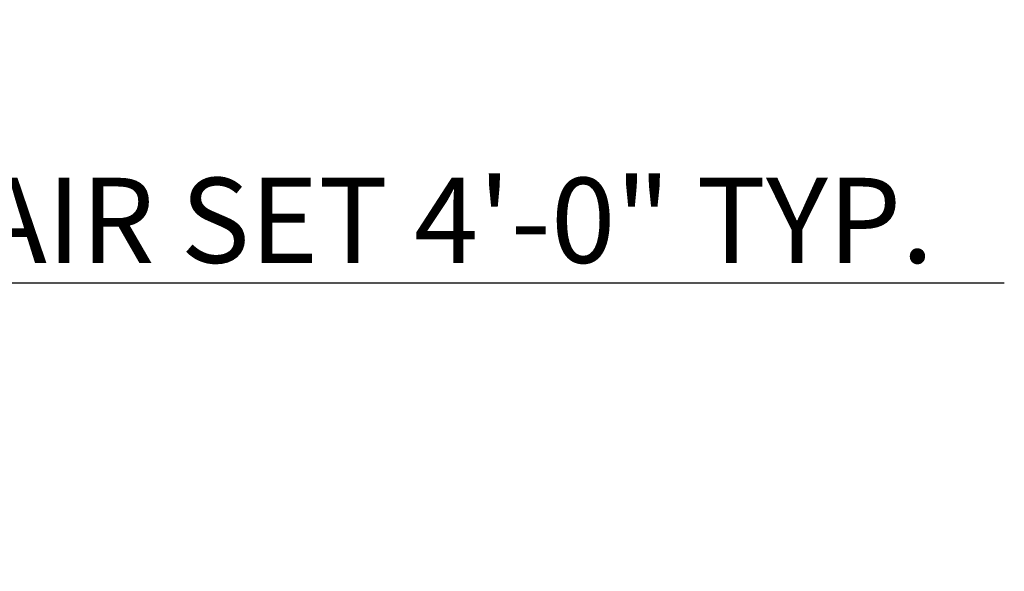
# Model space of a CAD drawing. Units: inches. Extents: x -7 to 1228, y -146 to 1091.
# Tile 16 of 88: x 420 to 501, y 12 to 57. Entities that reach past the tile are written whole.
import ezdxf

# ---------------------------------------------------------------- set-up
doc = ezdxf.new("R2010")
doc.units = ezdxf.units.IN
doc.layers.add('A-ANNO-DIMS', color=2, linetype='Continuous', lineweight=18)
doc.styles.get("Standard").update_dxf_attribs({"font": 'arial.ttf'})
doc.dimstyles.new('ISO-25', dxfattribs={"dimtxt": 7, "dimasz": 4, "dimexe": 1.25, "dimexo": 0.625, "dimtad": 1, "dimdec": 1, "dimlunit": 3, "dimtxsty": 'Standard', "dimcen": 2.5, "dimadec": 0, "dimazin": 0, "dimtfac": 1, "dimtdec": 1, "dimtmove": 1, "dimatfit": 3, "dimfxl": 1, "dimarcsym": 0})

# ---------------------------------------------------------------- blocks, each defined once
blk = doc.blocks.new('*D38')
at = {"layer": 'A-ANNO-DIMS', "color": 0, "lineweight": -2, "transparency": 16777216}
for p, q in [((324.905, 55.362), (324.905, 47.508)), ((373.098, 55.362), (373.098, 47.508)), ((328.905, 48.758), (369.098, 48.758)), ((349.002, 48.758), (352.917, 35.705)), ((352.917, 35.705), (500.857, 35.705))]:
    blk.add_line(p, q, dxfattribs=at)
at = {"layer": 'A-ANNO-DIMS', "color": 0, "transparency": 16777216}
for points in [[(328.905, 49.424), (328.905, 48.091), (324.905, 48.758)], [(369.098, 49.424), (369.098, 48.091), (373.098, 48.758)]]:
    blk.add_solid(points, dxfattribs=at)
at = {"layer": 'Defpoints', "color": 0, "transparency": 16777216}
for p in [(324.905, 55.987), (373.098, 55.987), (373.098, 48.758)]:
    blk.add_point(p, dxfattribs=at)
at = {"layer": 'A-ANNO-DIMS', "color": 0, "transparency": 16777216, "insert": (426.887, 39.952), "char_height": 7, "attachment_point": 5}
blk.add_mtext('BALCONY CHAIR SET 4\'-0" TYP.', dxfattribs=at)

msp = doc.modelspace()

# ---------------------------------------------------------------- dimensions: what is measured, and where the dimension line sits
at = {"layer": 'A-ANNO-DIMS'}
dim = msp.add_linear_dim(base=(373.098, 48.758), p1=(324.905, 55.987), p2=(373.098, 55.987), text='BALCONY CHAIR SET <> TYP.', dimstyle='ISO-25', override={"dimdec": 1, "dimlfac": 1, "dimrnd": 0, "dimzin": 1, "dimdsep": 46, "dimlunit": 4, "dimfrac": 2}, dxfattribs=at)
dim.commit()
dim.dimension.update_dxf_attribs({"geometry": '*D38', "text_midpoint": (353.542, 39.952)})

doc.saveas('drawing.dxf')
